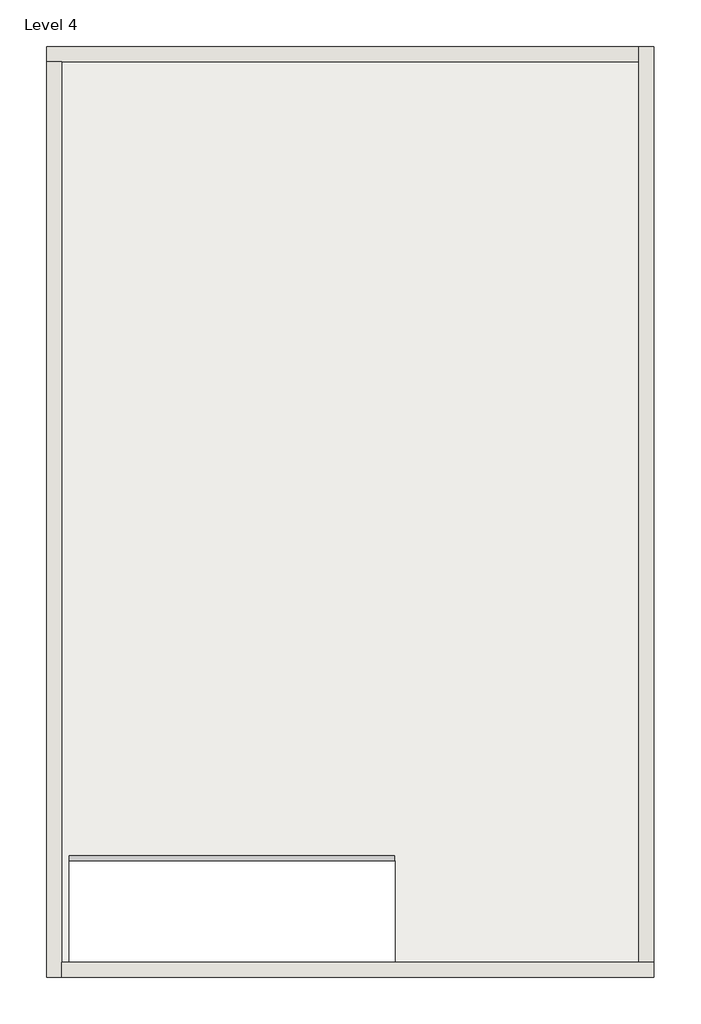
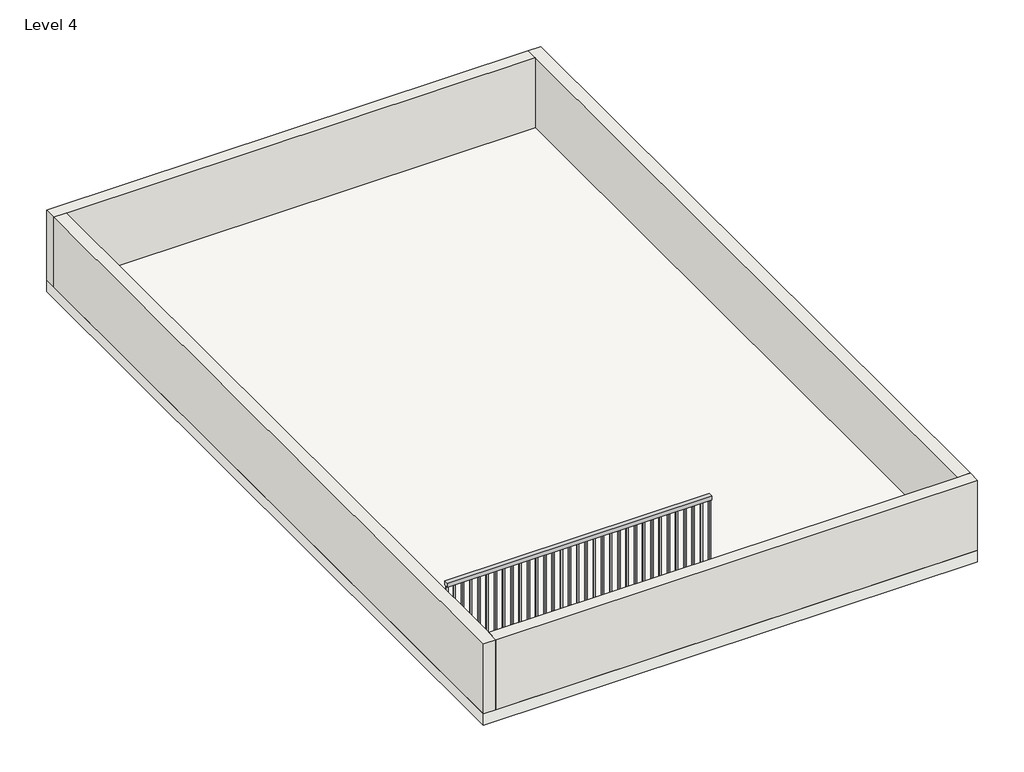
# One storey: 4 walls, 1 railing, 1 slab.
"""IFC4 building model written with IfcOpenShell, lengths in millimetres."""

from ifc_helpers import new_model, si_unit, frame, origin, place, context, project, spatial, polyline, outline, extrude, faceted_brep, element, save

model = new_model("IFC4")

# Units and contexts
model_context = context("Model", 3, world=origin())
ifc_project = project(units=[si_unit("LENGTHUNIT", "METRE", prefix="MILLI")], contexts=[model_context])

# Site, building, storey
site = spatial("IfcSite", under=ifc_project)
building = spatial("IfcBuilding", under=site)
storey = spatial("IfcBuildingStorey", under=building, Name="Level 4", Elevation=9601.2)

# Railing
placement = place(None, origin())
element("IfcRailing", 1, ObjectType="Handrail - Rectangular", at=placement, inside=storey, context=model_context, shape_type="SweptSolid", body=[
    extrude(outline(polyline([(-6471.1112714, -5835.257676), (-6471.1112714, -5784.457676), (-3209.2681702, -5784.457676), (-3209.2681702, -5835.257676), (-6471.1112714, -5835.257676)])), frame((0.0, 0.0, 10464.8), z_axis=(0.0, 0.0, 1.0), x_axis=(1.0, 0.0, 0.0)), (0.0, 0.0, 1.0), 50.8),
    extrude(outline(polyline([(-3229.4362714, -5819.382676), (-3229.4362714, -5800.332676), (-3210.3862714, -5800.332676), (-3210.3862714, -5819.382676), (-3229.4362714, -5819.382676)])), frame((0.0, 0.0, 9601.2), z_axis=(0.0, 0.0, 1.0), x_axis=(1.0, 0.0, 0.0)), (0.0, 0.0, 1.0), 863.6),
    extrude(outline(polyline([(-3331.0362714, -5819.382676), (-3331.0362714, -5800.332676), (-3311.9862714, -5800.332676), (-3311.9862714, -5819.382676), (-3331.0362714, -5819.382676)])), frame((0.0, 0.0, 9601.2), z_axis=(0.0, 0.0, 1.0), x_axis=(1.0, 0.0, 0.0)), (0.0, 0.0, 1.0), 863.6),
    extrude(outline(polyline([(-3432.6362714, -5819.382676), (-3432.6362714, -5800.332676), (-3413.5862714, -5800.332676), (-3413.5862714, -5819.382676), (-3432.6362714, -5819.382676)])), frame((0.0, 0.0, 9601.2), z_axis=(0.0, 0.0, 1.0), x_axis=(1.0, 0.0, 0.0)), (0.0, 0.0, 1.0), 863.6),
    extrude(outline(polyline([(-3534.2362714, -5819.382676), (-3534.2362714, -5800.332676), (-3515.1862714, -5800.332676), (-3515.1862714, -5819.382676), (-3534.2362714, -5819.382676)])), frame((0.0, 0.0, 9601.2), z_axis=(0.0, 0.0, 1.0), x_axis=(1.0, 0.0, 0.0)), (0.0, 0.0, 1.0), 863.6),
    extrude(outline(polyline([(-3635.8362714, -5819.382676), (-3635.8362714, -5800.332676), (-3616.7862714, -5800.332676), (-3616.7862714, -5819.382676), (-3635.8362714, -5819.382676)])), frame((0.0, 0.0, 9601.2), z_axis=(0.0, 0.0, 1.0), x_axis=(1.0, 0.0, 0.0)), (0.0, 0.0, 1.0), 863.6),
    extrude(outline(polyline([(-3737.4362714, -5819.382676), (-3737.4362714, -5800.332676), (-3718.3862714, -5800.332676), (-3718.3862714, -5819.382676), (-3737.4362714, -5819.382676)])), frame((0.0, 0.0, 9601.2), z_axis=(0.0, 0.0, 1.0), x_axis=(1.0, 0.0, 0.0)), (0.0, 0.0, 1.0), 863.6),
    extrude(outline(polyline([(-3839.0362714, -5819.382676), (-3839.0362714, -5800.332676), (-3819.9862714, -5800.332676), (-3819.9862714, -5819.382676), (-3839.0362714, -5819.382676)])), frame((0.0, 0.0, 9601.2), z_axis=(0.0, 0.0, 1.0), x_axis=(1.0, 0.0, 0.0)), (0.0, 0.0, 1.0), 863.6),
    extrude(outline(polyline([(-3940.6362714, -5819.382676), (-3940.6362714, -5800.332676), (-3921.5862714, -5800.332676), (-3921.5862714, -5819.382676), (-3940.6362714, -5819.382676)])), frame((0.0, 0.0, 9601.2), z_axis=(0.0, 0.0, 1.0), x_axis=(1.0, 0.0, 0.0)), (0.0, 0.0, 1.0), 863.6),
    extrude(outline(polyline([(-4042.2362714, -5819.382676), (-4042.2362714, -5800.332676), (-4023.1862714, -5800.332676), (-4023.1862714, -5819.382676), (-4042.2362714, -5819.382676)])), frame((0.0, 0.0, 9601.2), z_axis=(0.0, 0.0, 1.0), x_axis=(1.0, 0.0, 0.0)), (0.0, 0.0, 1.0), 863.6),
    extrude(outline(polyline([(-4143.8362714, -5819.382676), (-4143.8362714, -5800.332676), (-4124.7862714, -5800.332676), (-4124.7862714, -5819.382676), (-4143.8362714, -5819.382676)])), frame((0.0, 0.0, 9601.2), z_axis=(0.0, 0.0, 1.0), x_axis=(1.0, 0.0, 0.0)), (0.0, 0.0, 1.0), 863.6),
    extrude(outline(polyline([(-4245.4362714, -5819.382676), (-4245.4362714, -5800.332676), (-4226.3862714, -5800.332676), (-4226.3862714, -5819.382676), (-4245.4362714, -5819.382676)])), frame((0.0, 0.0, 9601.2), z_axis=(0.0, 0.0, 1.0), x_axis=(1.0, 0.0, 0.0)), (0.0, 0.0, 1.0), 863.6),
    extrude(outline(polyline([(-4347.0362714, -5819.382676), (-4347.0362714, -5800.332676), (-4327.9862714, -5800.332676), (-4327.9862714, -5819.382676), (-4347.0362714, -5819.382676)])), frame((0.0, 0.0, 9601.2), z_axis=(0.0, 0.0, 1.0), x_axis=(1.0, 0.0, 0.0)), (0.0, 0.0, 1.0), 863.6),
    extrude(outline(polyline([(-4448.6362714, -5819.382676), (-4448.6362714, -5800.332676), (-4429.5862714, -5800.332676), (-4429.5862714, -5819.382676), (-4448.6362714, -5819.382676)])), frame((0.0, 0.0, 9601.2), z_axis=(0.0, 0.0, 1.0), x_axis=(1.0, 0.0, 0.0)), (0.0, 0.0, 1.0), 863.6),
    extrude(outline(polyline([(-4550.2362714, -5819.382676), (-4550.2362714, -5800.332676), (-4531.1862714, -5800.332676), (-4531.1862714, -5819.382676), (-4550.2362714, -5819.382676)])), frame((0.0, 0.0, 9601.2), z_axis=(0.0, 0.0, 1.0), x_axis=(1.0, 0.0, 0.0)), (0.0, 0.0, 1.0), 863.6),
    extrude(outline(polyline([(-4651.8362714, -5819.382676), (-4651.8362714, -5800.332676), (-4632.7862714, -5800.332676), (-4632.7862714, -5819.382676), (-4651.8362714, -5819.382676)])), frame((0.0, 0.0, 9601.2), z_axis=(0.0, 0.0, 1.0), x_axis=(1.0, 0.0, 0.0)), (0.0, 0.0, 1.0), 863.6),
    extrude(outline(polyline([(-4753.4362714, -5819.382676), (-4753.4362714, -5800.332676), (-4734.3862714, -5800.332676), (-4734.3862714, -5819.382676), (-4753.4362714, -5819.382676)])), frame((0.0, 0.0, 9601.2), z_axis=(0.0, 0.0, 1.0), x_axis=(1.0, 0.0, 0.0)), (0.0, 0.0, 1.0), 863.6),
    extrude(outline(polyline([(-4855.0362714, -5819.382676), (-4855.0362714, -5800.332676), (-4835.9862714, -5800.332676), (-4835.9862714, -5819.382676), (-4855.0362714, -5819.382676)])), frame((0.0, 0.0, 9601.2), z_axis=(0.0, 0.0, 1.0), x_axis=(1.0, 0.0, 0.0)), (0.0, 0.0, 1.0), 863.6),
    extrude(outline(polyline([(-4956.6362714, -5819.382676), (-4956.6362714, -5800.332676), (-4937.5862714, -5800.332676), (-4937.5862714, -5819.382676), (-4956.6362714, -5819.382676)])), frame((0.0, 0.0, 9601.2), z_axis=(0.0, 0.0, 1.0), x_axis=(1.0, 0.0, 0.0)), (0.0, 0.0, 1.0), 863.6),
    extrude(outline(polyline([(-5058.2362714, -5819.382676), (-5058.2362714, -5800.332676), (-5039.1862714, -5800.332676), (-5039.1862714, -5819.382676), (-5058.2362714, -5819.382676)])), frame((0.0, 0.0, 9601.2), z_axis=(0.0, 0.0, 1.0), x_axis=(1.0, 0.0, 0.0)), (0.0, 0.0, 1.0), 863.6),
    extrude(outline(polyline([(-5159.8362714, -5819.382676), (-5159.8362714, -5800.332676), (-5140.7862714, -5800.332676), (-5140.7862714, -5819.382676), (-5159.8362714, -5819.382676)])), frame((0.0, 0.0, 9601.2), z_axis=(0.0, 0.0, 1.0), x_axis=(1.0, 0.0, 0.0)), (0.0, 0.0, 1.0), 863.6),
    extrude(outline(polyline([(-5261.4362714, -5819.382676), (-5261.4362714, -5800.332676), (-5242.3862714, -5800.332676), (-5242.3862714, -5819.382676), (-5261.4362714, -5819.382676)])), frame((0.0, 0.0, 9601.2), z_axis=(0.0, 0.0, 1.0), x_axis=(1.0, 0.0, 0.0)), (0.0, 0.0, 1.0), 863.6),
    extrude(outline(polyline([(-5363.0362714, -5819.382676), (-5363.0362714, -5800.332676), (-5343.9862714, -5800.332676), (-5343.9862714, -5819.382676), (-5363.0362714, -5819.382676)])), frame((0.0, 0.0, 9601.2), z_axis=(0.0, 0.0, 1.0), x_axis=(1.0, 0.0, 0.0)), (0.0, 0.0, 1.0), 863.6),
    extrude(outline(polyline([(-5464.6362714, -5819.382676), (-5464.6362714, -5800.332676), (-5445.5862714, -5800.332676), (-5445.5862714, -5819.382676), (-5464.6362714, -5819.382676)])), frame((0.0, 0.0, 9601.2), z_axis=(0.0, 0.0, 1.0), x_axis=(1.0, 0.0, 0.0)), (0.0, 0.0, 1.0), 863.6),
    extrude(outline(polyline([(-5566.2362714, -5819.382676), (-5566.2362714, -5800.332676), (-5547.1862714, -5800.332676), (-5547.1862714, -5819.382676), (-5566.2362714, -5819.382676)])), frame((0.0, 0.0, 9601.2), z_axis=(0.0, 0.0, 1.0), x_axis=(1.0, 0.0, 0.0)), (0.0, 0.0, 1.0), 863.6),
    extrude(outline(polyline([(-5667.8362714, -5819.382676), (-5667.8362714, -5800.332676), (-5648.7862714, -5800.332676), (-5648.7862714, -5819.382676), (-5667.8362714, -5819.382676)])), frame((0.0, 0.0, 9601.2), z_axis=(0.0, 0.0, 1.0), x_axis=(1.0, 0.0, 0.0)), (0.0, 0.0, 1.0), 863.6),
    extrude(outline(polyline([(-5769.4362714, -5819.382676), (-5769.4362714, -5800.332676), (-5750.3862714, -5800.332676), (-5750.3862714, -5819.382676), (-5769.4362714, -5819.382676)])), frame((0.0, 0.0, 9601.2), z_axis=(0.0, 0.0, 1.0), x_axis=(1.0, 0.0, 0.0)), (0.0, 0.0, 1.0), 863.6),
    extrude(outline(polyline([(-5871.0362714, -5819.382676), (-5871.0362714, -5800.332676), (-5851.9862714, -5800.332676), (-5851.9862714, -5819.382676), (-5871.0362714, -5819.382676)])), frame((0.0, 0.0, 9601.2), z_axis=(0.0, 0.0, 1.0), x_axis=(1.0, 0.0, 0.0)), (0.0, 0.0, 1.0), 863.6),
    extrude(outline(polyline([(-5972.6362714, -5819.382676), (-5972.6362714, -5800.332676), (-5953.5862714, -5800.332676), (-5953.5862714, -5819.382676), (-5972.6362714, -5819.382676)])), frame((0.0, 0.0, 9601.2), z_axis=(0.0, 0.0, 1.0), x_axis=(1.0, 0.0, 0.0)), (0.0, 0.0, 1.0), 863.6),
    extrude(outline(polyline([(-6074.2362714, -5819.382676), (-6074.2362714, -5800.332676), (-6055.1862714, -5800.332676), (-6055.1862714, -5819.382676), (-6074.2362714, -5819.382676)])), frame((0.0, 0.0, 9601.2), z_axis=(0.0, 0.0, 1.0), x_axis=(1.0, 0.0, 0.0)), (0.0, 0.0, 1.0), 863.6),
    extrude(outline(polyline([(-6175.8362714, -5819.382676), (-6175.8362714, -5800.332676), (-6156.7862714, -5800.332676), (-6156.7862714, -5819.382676), (-6175.8362714, -5819.382676)])), frame((0.0, 0.0, 9601.2), z_axis=(0.0, 0.0, 1.0), x_axis=(1.0, 0.0, 0.0)), (0.0, 0.0, 1.0), 863.6),
    extrude(outline(polyline([(-6277.4362714, -5819.382676), (-6277.4362714, -5800.332676), (-6258.3862714, -5800.332676), (-6258.3862714, -5819.382676), (-6277.4362714, -5819.382676)])), frame((0.0, 0.0, 9601.2), z_axis=(0.0, 0.0, 1.0), x_axis=(1.0, 0.0, 0.0)), (0.0, 0.0, 1.0), 863.6),
    extrude(outline(polyline([(-6379.0362714, -5819.382676), (-6379.0362714, -5800.332676), (-6359.9862714, -5800.332676), (-6359.9862714, -5819.382676), (-6379.0362714, -5819.382676)])), frame((0.0, 0.0, 9601.2), z_axis=(0.0, 0.0, 1.0), x_axis=(1.0, 0.0, 0.0)), (0.0, 0.0, 1.0), 863.6),
    extrude(outline(polyline([(-3228.3181702, -5819.382676), (-3228.3181702, -5800.332676), (-3209.2681702, -5800.332676), (-3209.2681702, -5819.382676), (-3228.3181702, -5819.382676)])), frame((0.0, 0.0, 9601.2), z_axis=(0.0, 0.0, 1.0), x_axis=(1.0, 0.0, 0.0)), (0.0, 0.0, 1.0), 863.6),
    extrude(outline(polyline([(-6471.1112714, -5819.382676), (-6471.1112714, -5800.332676), (-6452.0612714, -5800.332676), (-6452.0612714, -5819.382676), (-6471.1112714, -5819.382676)])), frame((0.0, 0.0, 9601.2), z_axis=(0.0, 0.0, 1.0), x_axis=(1.0, 0.0, 0.0)), (0.0, 0.0, 1.0), 863.6),
])

# Slab
element("IfcSlab", 2, ObjectType="6\"", at=placement, inside=storey, context=model_context, shape_type="SweptSolid", body=[
    extrude(outline(polyline([(-603.7112714, 2330.842324), (-603.7112714, -7003.657676), (-6699.7112714, -7003.657676), (-6699.7112714, 2330.842324), (-603.7112714, 2330.842324)]), holes=[polyline([(-6471.1112714, -6851.257676), (-3204.6473712, -6851.257676), (-3204.6473712, -5835.257676), (-6471.1112714, -5835.257676), (-6471.1112714, -6851.257676)])]), frame((0.0, 0.0, 9448.8), z_axis=(0.0, 0.0, 1.0), x_axis=(1.0, 0.0, 0.0)), (0.0, 0.0, 1.0), 152.4),
])

# Walls
element("IfcWall", 3, ObjectType="6\"", at=placement, inside=storey, context=model_context, shape_type="Brep", body=[
    faceted_brep([(-6699.7112714, 2178.442324, 9601.2), (-6547.3112714, 2178.442324, 9601.2), (-756.1112714, 2178.442324, 9601.2), (-756.1112714, 2178.442324, 10515.6), (-6547.3112714, 2178.442324, 10515.6), (-6699.7112714, 2178.442324, 10515.6), (-6699.7112714, 2330.842324, 9601.2), (-6699.7112714, 2330.842324, 10515.6), (-756.1112714, 2330.842324, 10515.6), (-756.1112714, 2330.842324, 9601.2)], [[[0, 1, 2, 3, 4, 5]], [[6, 7, 8, 9]], [[2, 1, 0, 6, 9]], [[5, 4, 3, 8, 7]], [[0, 5, 7, 6]], [[3, 2, 9, 8]]]),
])
element("IfcWall", 4, ObjectType="6\"", at=placement, inside=storey, context=model_context, shape_type="Brep", body=[
    faceted_brep([(-6547.3112714, -7003.657676, 9601.2), (-6547.3112714, -6851.257676, 9601.2), (-6547.3112714, 2178.442324, 9601.2), (-6547.3112714, 2178.442324, 10515.6), (-6547.3112714, -6851.257676, 10515.6), (-6547.3112714, -7003.657676, 10515.6), (-6699.7112714, -7003.657676, 9601.2), (-6699.7112714, -7003.657676, 10515.6), (-6699.7112714, 2178.442324, 10515.6), (-6699.7112714, 2178.442324, 9601.2)], [[[0, 1, 2, 3, 4, 5]], [[6, 7, 8, 9]], [[2, 1, 0, 6, 9]], [[5, 4, 3, 8, 7]], [[0, 5, 7, 6]], [[3, 2, 9, 8]]]),
])
element("IfcWall", 5, ObjectType="6\"", at=placement, inside=storey, context=model_context, shape_type="Brep", body=[
    faceted_brep([(-603.7112714, -6851.257676, 9601.2), (-756.1112714, -6851.257676, 9601.2), (-6547.3112714, -6851.257676, 9601.2), (-6547.3112714, -6851.257676, 10515.6), (-756.1112714, -6851.257676, 10515.6), (-603.7112714, -6851.257676, 10515.6), (-603.7112714, -7003.657676, 9601.2), (-603.7112714, -7003.657676, 10515.6), (-6547.3112714, -7003.657676, 10515.6), (-6547.3112714, -7003.657676, 9601.2)], [[[0, 1, 2, 3, 4, 5]], [[6, 7, 8, 9]], [[2, 1, 0, 6, 9]], [[5, 4, 3, 8, 7]], [[0, 5, 7, 6]], [[3, 2, 9, 8]]]),
])
element("IfcWall", 6, ObjectType="6\"", at=placement, inside=storey, context=model_context, shape_type="Brep", body=[
    faceted_brep([(-756.1112714, 2330.842324, 9601.2), (-756.1112714, 2178.442324, 9601.2), (-756.1112714, -6851.257676, 9601.2), (-756.1112714, -6851.257676, 10515.6), (-756.1112714, 2178.442324, 10515.6), (-756.1112714, 2330.842324, 10515.6), (-603.7112714, 2330.842324, 9601.2), (-603.7112714, 2330.842324, 10515.6), (-603.7112714, -6851.257676, 10515.6), (-603.7112714, -6851.257676, 9601.2)], [[[0, 1, 2, 3, 4, 5]], [[6, 7, 8, 9]], [[2, 1, 0, 6, 9]], [[5, 4, 3, 8, 7]], [[0, 5, 7, 6]], [[3, 2, 9, 8]]]),
])

save(model, "model.ifc")

# Revit data of these elements
# Type "Handrail - Rectangular"
#   Assembly Code = "C2010400"
#   built-in parameter 1008612 = 0.0416667 (stored number, unit not read)
#   built-in parameter 1008611 = 0.0416667 (stored number, unit not read)
#   built-in parameter 1008609 = 0.333333 (stored number, unit not read)
#   built-in parameter 1008604 = 0.166667 (stored number, unit not read)
#   built-in parameter 1008603 = 0.166667 (stored number, unit not read)
#   Railing Height = 3' - 0"
#   built-in parameter 1008630 = 2
#   built-in parameter 1008610 = 2
#   built-in parameter 1008618 = Baluster - Square : 3/4"
# Type "6\""
#   Assembly Code = "B1010"
#   Function = 0
#   Layers, outside or top first: 0' - 6" "floor" (function 1)
# Type "6\""
#   Assembly Code = "B2010"
#   Layers, outside or top first: 0' - 6" "ext wall" (function 1)
# Element 1 (IfcRailing, "Handrail - Rectangular")
#   Phase Created = New Construction
# Element 2 (IfcSlab, "6\"")
#   Height Offset From Level = 0' - 0"
#   Phase Created = New Construction
#   Materials on its faces: "floor"
# Elements 3, 4, 5, 6 (IfcWall, "6\"")
#   Top Offset = 0' - 0"
#   Base Offset = 0' - 0"
#   Unconnected Height = 3' - 0"
#   wall height = 3' - 0"
#   Phase Created = New Construction
#   Base Constraint = Level 4
#   Materials on its faces: "ext wall"
# Materials
#   "floor": class "Generic", colour RGB 138 129 123, transparency 0, Cost = 0
#   "ext wall": class "Generic", colour RGB 219 210 180, transparency 0, Cost = 0
